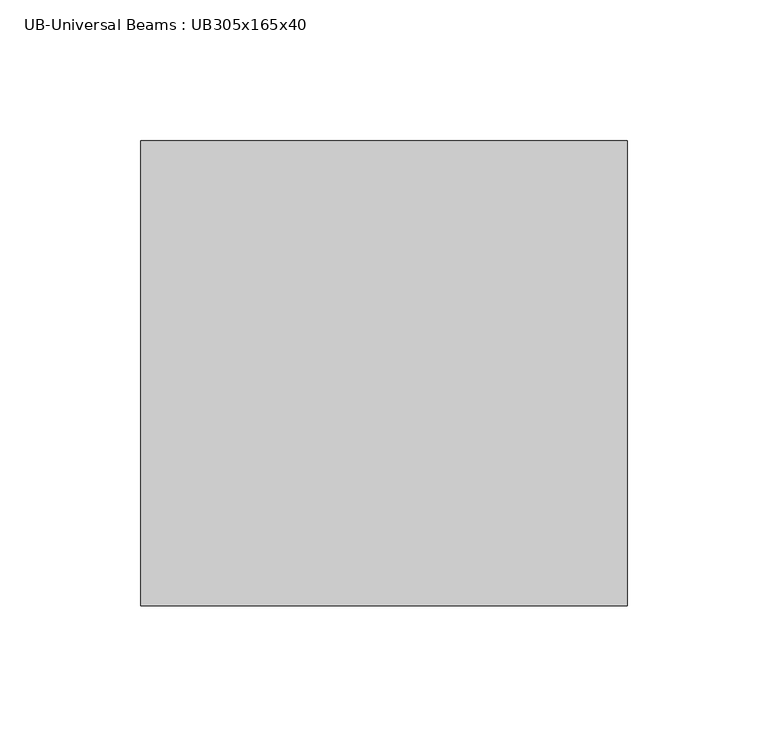
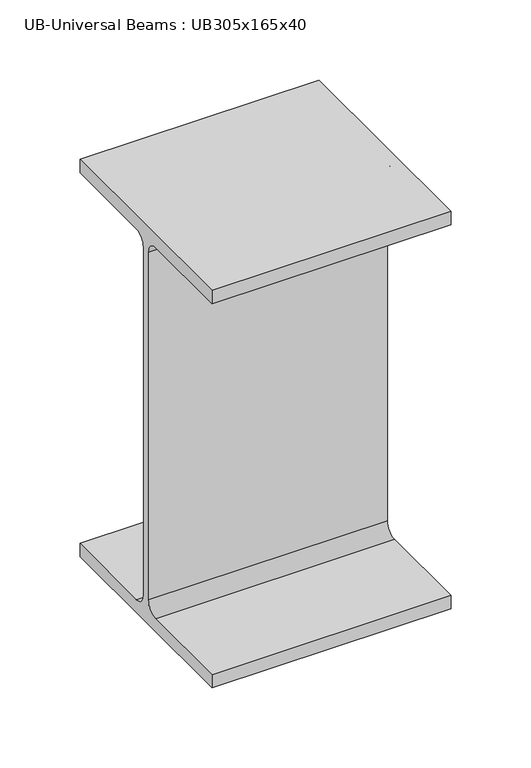
"""IFC4 building model written with IfcOpenShell, lengths in millimetres: beam geometry, UB-Universal Beams : UB305x165x40."""

from ifc_helpers import new_model, si_unit, point, frame, frame_2d, origin, place, context, project, spatial, polyline, circle_curve, trimmed, segment, composite_curve, outline, extrude, source, transform, mapped, element, save


def ub_universal_beams_ub305x165x40_52a2f76b(model_context):
    return source(origin(), model_context, "Body", "SweptSolid", [
        extrude(outline(composite_curve([segment(polyline([(82.5, -141.5), (82.5, -151.7), (-82.5, -151.7), (-82.5, -141.5), (-11.9, -141.5)]), True, "CONTINUOUS"), segment(trimmed(circle_curve(frame_2d((-11.9, -132.6)), 8.9), [point((-11.9, -141.5))], [point((-3.0, -132.6))], True, "CARTESIAN"), True, "CONTINUOUS"), segment(polyline([(-3.0, -132.6), (-3.0, 132.6)]), True, "CONTINUOUS"), segment(trimmed(circle_curve(frame_2d((-11.9, 132.6)), 8.9), [point((-3.0, 132.6))], [point((-11.9, 141.5))], True, "CARTESIAN"), True, "CONTINUOUS"), segment(polyline([(-11.9, 141.5), (-82.5, 141.5), (-82.5, 151.7), (82.5, 151.7), (82.5, 141.5), (11.9, 141.5)]), True, "CONTINUOUS"), segment(trimmed(circle_curve(frame_2d((11.9, 132.6)), 8.9), [point((11.9, 141.5))], [point((3.0, 132.6))], True, "CARTESIAN"), True, "CONTINUOUS"), segment(polyline([(3.0, 132.6), (3.0, -132.6)]), True, "CONTINUOUS"), segment(trimmed(circle_curve(frame_2d((11.9, -132.6)), 8.9), [point((3.0, -132.6))], [point((11.9, -141.5))], True, "CARTESIAN"), True, "CONTINUOUS"), segment(polyline([(11.9, -141.5), (82.5, -141.5)]), True, "CONTINUOUS")], self_intersect=False)), frame((-111.75, 0.0, 0.0), z_axis=(1.0, 0.0, 0.0), x_axis=(0.0, 1.0, 0.0)), (0.0, 0.0, 1.0), 172.6),
    ])


if __name__ == "__main__":
    model = new_model("IFC4")
    model_context = context("Model", 3, world=origin())
    ifc_project = project(units=[si_unit("LENGTHUNIT", "METRE", prefix="MILLI")], contexts=[model_context])
    site = spatial("IfcSite", under=ifc_project)
    building = spatial("IfcBuilding", under=site)
    placement = place(None, origin())
    ub_universal_beams_ub305x165x40_shape = ub_universal_beams_ub305x165x40_52a2f76b(model_context)
    element("IfcBeam", 1, ObjectType="UB-Universal Beams : UB305x165x40", at=placement, inside=building, context=model_context, shape_type="MappedRepresentation", body=[
        mapped(ub_universal_beams_ub305x165x40_shape, transform((0.0, 0.0, 0.0), x_axis=(1.0, 0.0, 0.0), y_axis=(0.0, 1.0, 0.0), z_axis=(0.0, 0.0, 1.0))),
    ])
    save(model, "model.ifc")

# Revit data of these elements
# Type "UB-Universal Beams : UB305x165x40"
#   Section Name Key = "UB305X165X40"
#   Width = 16.5 cm
#   Web Thickness = 0.6 cm
#   Web Fillet = 0.89 cm
#   Warping Constant = 164000.0 cm⁶
#   Torsional Moment of Inertia = 14.70 cm⁴
#   Section Area = 51.3 cm²
#   Plastic Modulus weak axis = 142.0 cm³
#   Plastic Modulus strong axis = 623.0 cm³
#   Nominal Weight = 40.2999 kgf/m
#   Moment of Inertia weak axis = 764.00 cm⁴
#   Moment of Inertia strong axis = 8503.00 cm⁴
#   Height = 30.34 cm
#   Flange Thickness = 1.02 cm
#   Elastic Modulus weak axis = 92.6 cm³
#   Elastic Modulus strong axis = 560.0 cm³
#   Centroid Vertical = 15.17 cm
#   Centroid Horizontal = 8.25 cm
#   Bolt Spacing = 9.0 cm
#   Length [instance default] = 1500 mm
#   Structural Material [instance default] = Metal - Steel 43-275
#   Type Comments = ""
#   Assembly Code = ""
# Element 1 (IfcBeam, "UB-Universal Beams : UB305x165x40")
#   Materials on its faces: "Metal - Steel 43-275"
# Materials
#   "Metal - Steel 43-275": class "Metal", colour RGB 247 247 247, transparency 0, Cost = 0
